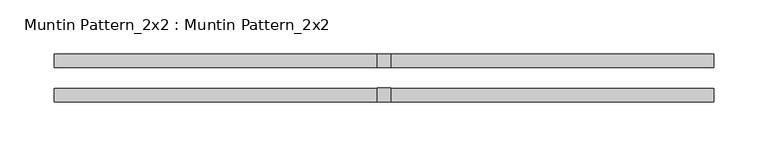
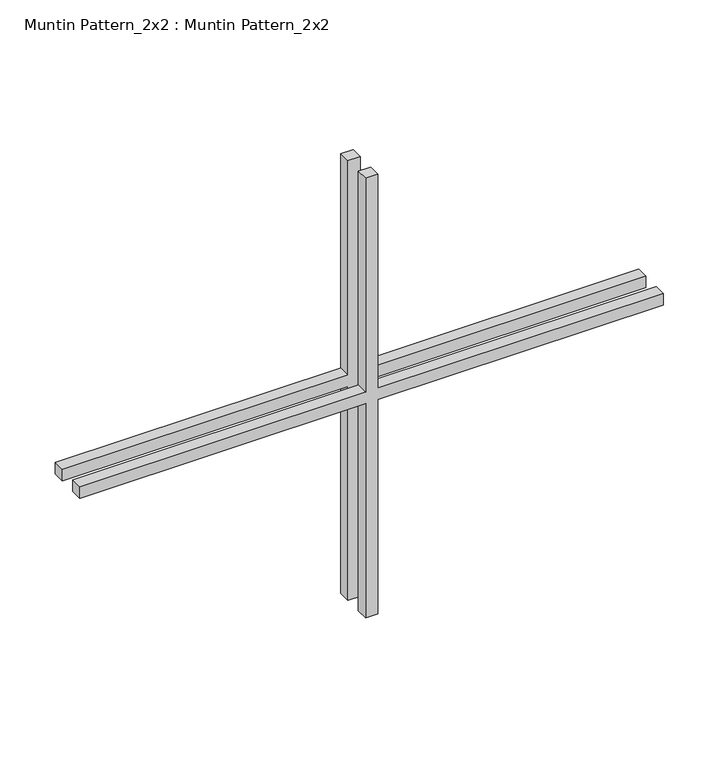
"""IFC4 building model written with IfcOpenShell, lengths in millimetres: proxy geometry, Muntin Pattern_2x2 : Muntin Pattern_2x2."""

from ifc_helpers import new_model, si_unit, frame, origin, place, context, project, spatial, polyline, outline, extrude, source, transform, mapped, element, save


def muntin_pattern_2x2_muntin_pattern_2x2_b8ba09c9(model_context):
    return source(origin(), model_context, "Body", "SweptSolid", [
        extrude(outline(polyline([(249.2375, -6.35), (249.2375, -304.8), (236.5375, -304.8), (236.5375, -6.35), (0.0, -6.35), (0.0, 6.35), (236.5375, 6.35), (236.5375, 304.8), (249.2375, 304.8), (249.2375, 6.35), (485.775, 6.35), (485.775, -6.35), (249.2375, -6.35)])), frame((0.0, 9.525, 0.0), z_axis=(0.0, 1.0, 0.0), x_axis=(0.0, 0.0, 1.0)), (0.0, 0.0, 1.0), 12.7),
        extrude(outline(polyline([(249.2375, -6.35), (249.2375, -304.8), (236.5375, -304.8), (236.5375, -6.35), (0.0, -6.35), (0.0, 6.35), (236.5375, 6.35), (236.5375, 304.8), (249.2375, 304.8), (249.2375, 6.35), (485.775, 6.35), (485.775, -6.35), (249.2375, -6.35)])), frame((0.0, -22.225, 0.0), z_axis=(0.0, 1.0, 0.0), x_axis=(0.0, 0.0, 1.0)), (0.0, 0.0, 1.0), 12.7),
    ])


if __name__ == "__main__":
    model = new_model("IFC4")
    model_context = context("Model", 3, world=origin())
    ifc_project = project(units=[si_unit("LENGTHUNIT", "METRE", prefix="MILLI")], contexts=[model_context])
    site = spatial("IfcSite", under=ifc_project)
    building = spatial("IfcBuilding", under=site)
    placement = place(None, origin())
    muntin_pattern_2x2_muntin_pattern_2x2_shape = muntin_pattern_2x2_muntin_pattern_2x2_b8ba09c9(model_context)
    element("IfcBuildingElementProxy", 1, Name="Muntin Pattern_2x2 : Muntin Pattern_2x2", ObjectType="Muntin Pattern_2x2 : Muntin Pattern_2x2", at=placement, inside=building, context=model_context, shape_type="MappedRepresentation", body=[
        mapped(muntin_pattern_2x2_muntin_pattern_2x2_shape, transform((0.0, 0.0, 0.0), x_axis=(1.0, 0.0, 0.0), y_axis=(0.0, 1.0, 0.0), z_axis=(0.0, 0.0, 1.0))),
    ])
    save(model, "model.ifc")

# Revit data of these elements
# Type "Muntin Pattern_2x2 : Muntin Pattern_2x2"
#   Width [instance default] = 4' - 0"
#   Thickness = 0' - 0 1/2"
#   Height [instance default] = 4' - 0"
#   Distance = 0' - 0 3/4"
#   Interior Material [instance default] = none
#   Exterior Material [instance default] = none
#   Default Elevation = 0
# Element 1 (IfcBuildingElementProxy, "Muntin Pattern_2x2 : Muntin Pattern_2x2")
#   Width = 2' - 0"
#   Height = 1' - 7 1/8"
#   Interior Material = Wood - Stained
#   Exterior Material = Clad - White
#   Materials on its faces: "Clad - White", "Wood - Stained"
# Materials
#   "Clad - White": class "Wood", colour RGB 242 242 238, transparency 0, Cost = 0
#   "Wood - Stained": class "Wood", colour RGB 224 178 126, transparency 0, Cost = 0
